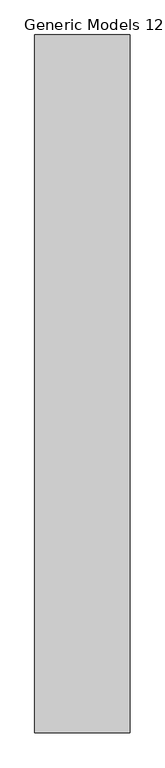
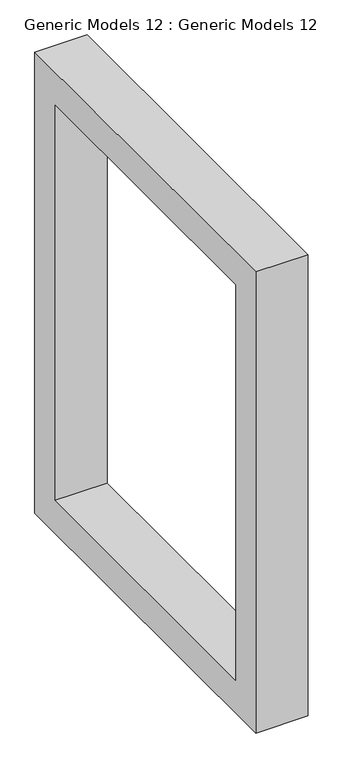
"""IFC4 building model written with IfcOpenShell, lengths in millimetres: proxy geometry, Generic Models 12 : Generic Models 12."""

from ifc_helpers import new_model, si_unit, frame, origin, place, context, project, spatial, polyline, outline, extrude, source, transform, mapped, element, save


def generic_models_12_generic_models_12_5399d40d(model_context):
    return source(origin(), model_context, "Body", "SweptSolid", [
        extrude(outline(polyline([(4025.9641252, 6305.8433359), (5143.5641252, 6305.8433359), (5143.5641252, 4883.4433359), (4025.9641252, 4883.4433359), (4025.9641252, 6305.8433359)]), holes=[polyline([(4127.5641252, 6204.2433359), (4127.5641252, 4985.0433359), (5041.9641252, 4985.0433359), (5041.9641252, 6204.2433359), (4127.5641252, 6204.2433359)])]), frame((-6249.7932997, 0.0, 0.0), z_axis=(1.0, 0.0, 0.0), x_axis=(0.0, 1.0, 0.0)), (0.0, 0.0, 1.0), 152.4),
    ])


if __name__ == "__main__":
    model = new_model("IFC4")
    model_context = context("Model", 3, world=origin())
    ifc_project = project(units=[si_unit("LENGTHUNIT", "METRE", prefix="MILLI")], contexts=[model_context])
    site = spatial("IfcSite", under=ifc_project)
    building = spatial("IfcBuilding", under=site)
    placement = place(None, origin())
    generic_models_12_generic_models_12_shape = generic_models_12_generic_models_12_5399d40d(model_context)
    element("IfcBuildingElementProxy", 1, Name="Generic Models 12 : Generic Models 12", ObjectType="Generic Models 12 : Generic Models 12", at=placement, inside=building, context=model_context, shape_type="MappedRepresentation", body=[
        mapped(generic_models_12_generic_models_12_shape, transform((0.0, 0.0, 0.0), x_axis=(1.0, 0.0, 0.0), y_axis=(0.0, 1.0, 0.0), z_axis=(0.0, 0.0, 1.0))),
    ])
    save(model, "model.ifc")

# Revit data of these elements
# Element 1 (IfcBuildingElementProxy, "Generic Models 12 : Generic Models 12")
#   Materials on its faces: "chocolate brown"
# Materials
#   "chocolate brown": class "Generic", colour RGB 120 120 120, transparency 0, Cost = 0
